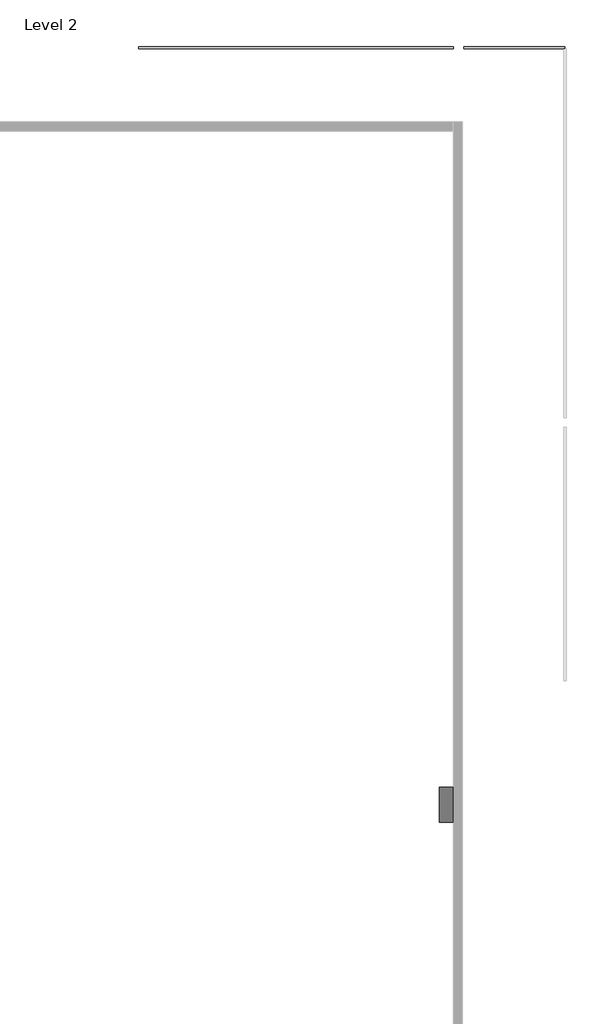
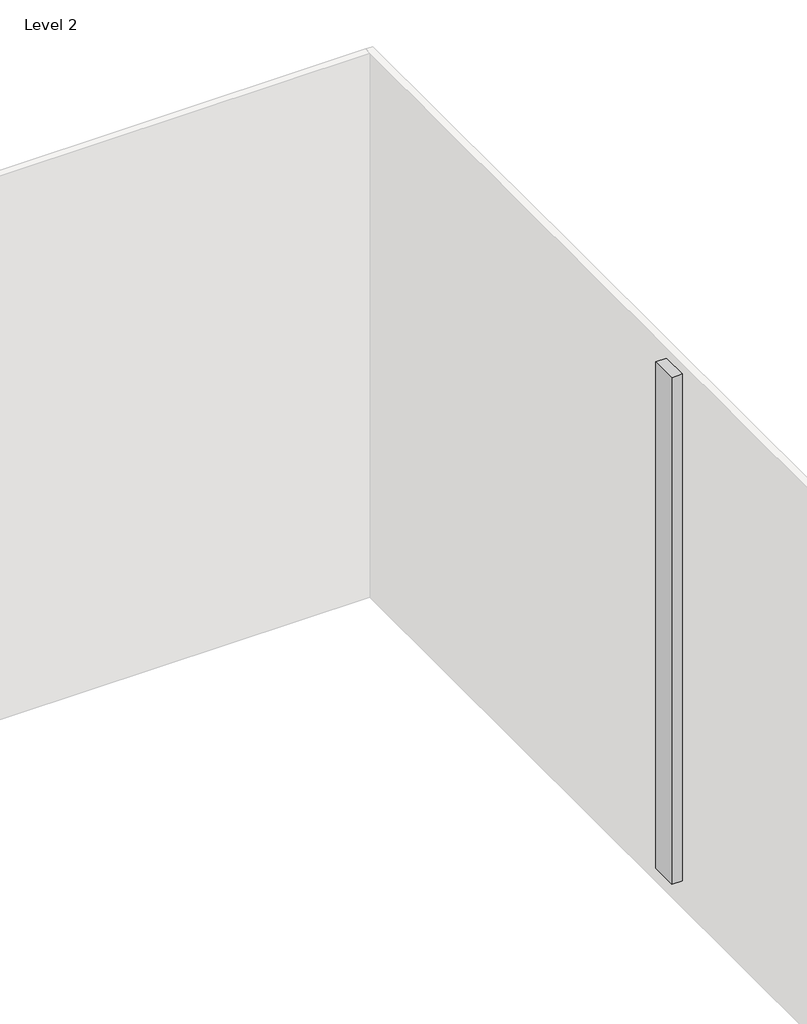
# One storey, part 5 of 5: 2 railings, 1 proxy.
"""IFC4 building model written with IfcOpenShell, lengths in millimetres."""

from ifc_helpers import new_model, si_unit, frame, origin, place, context, project, spatial, polyline, outline, extrude, transform, mapped, element, save
from components import generic_models_2_generic_models_2_fd6437b6

model = new_model("IFC4")

# Units and contexts
model_context = context("Model", 3, world=origin())
ifc_project = project(units=[si_unit("LENGTHUNIT", "METRE", prefix="MILLI")], contexts=[model_context])

# Site, building, storey
site = spatial("IfcSite", under=ifc_project)
building = spatial("IfcBuilding", under=site)
storey = spatial("IfcBuildingStorey", under=building, Name="Level 2", Elevation=3048.0)

# Proxy
placement = place(None, origin())
generic_models_2_generic_models_2_shape = generic_models_2_generic_models_2_fd6437b6(model_context)
element("IfcBuildingElementProxy", 1, Name="Generic Models 2 : Generic Models 2", ObjectType="Generic Models 2 : Generic Models 2", at=placement, inside=storey, context=model_context, shape_type="MappedRepresentation", body=[
    mapped(generic_models_2_generic_models_2_shape, transform((0.0, 0.0, 0.0), x_axis=(1.0, 0.0, 0.0), y_axis=(0.0, 1.0, 0.0), z_axis=(0.0, 0.0, 1.0))),
])

# Railings
element("IfcRailing", 2, ObjectType="Handrail - Rectangular", at=placement, inside=storey, context=model_context, shape_type="SweptSolid", body=[
    extrude(outline(polyline([(14131.9361222, 16349.0250499), (14131.9361222, 16399.8250499), (16321.4289933, 16399.8250499), (16321.4289933, 16349.0250499), (14131.9361222, 16349.0250499)])), frame((0.0, 0.0, 3911.6), z_axis=(0.0, 0.0, 1.0), x_axis=(1.0, 0.0, 0.0)), (0.0, 0.0, 1.0), 50.8),
    extrude(outline(polyline([(16256.0111222, 16364.9000499), (16256.0111222, 16383.9500499), (16275.0611222, 16383.9500499), (16275.0611222, 16364.9000499), (16256.0111222, 16364.9000499)])), frame((0.0, 0.0, 3048.0), z_axis=(0.0, 0.0, 1.0), x_axis=(1.0, 0.0, 0.0)), (0.0, 0.0, 1.0), 863.6),
    extrude(outline(polyline([(16154.4111222, 16364.9000499), (16154.4111222, 16383.9500499), (16173.4611222, 16383.9500499), (16173.4611222, 16364.9000499), (16154.4111222, 16364.9000499)])), frame((0.0, 0.0, 3048.0), z_axis=(0.0, 0.0, 1.0), x_axis=(1.0, 0.0, 0.0)), (0.0, 0.0, 1.0), 863.6),
    extrude(outline(polyline([(16052.8111222, 16364.9000499), (16052.8111222, 16383.9500499), (16071.8611222, 16383.9500499), (16071.8611222, 16364.9000499), (16052.8111222, 16364.9000499)])), frame((0.0, 0.0, 3048.0), z_axis=(0.0, 0.0, 1.0), x_axis=(1.0, 0.0, 0.0)), (0.0, 0.0, 1.0), 863.6),
    extrude(outline(polyline([(15951.2111222, 16364.9000499), (15951.2111222, 16383.9500499), (15970.2611222, 16383.9500499), (15970.2611222, 16364.9000499), (15951.2111222, 16364.9000499)])), frame((0.0, 0.0, 3048.0), z_axis=(0.0, 0.0, 1.0), x_axis=(1.0, 0.0, 0.0)), (0.0, 0.0, 1.0), 863.6),
    extrude(outline(polyline([(15849.6111222, 16364.9000499), (15849.6111222, 16383.9500499), (15868.6611222, 16383.9500499), (15868.6611222, 16364.9000499), (15849.6111222, 16364.9000499)])), frame((0.0, 0.0, 3048.0), z_axis=(0.0, 0.0, 1.0), x_axis=(1.0, 0.0, 0.0)), (0.0, 0.0, 1.0), 863.6),
    extrude(outline(polyline([(15748.0111222, 16364.9000499), (15748.0111222, 16383.9500499), (15767.0611222, 16383.9500499), (15767.0611222, 16364.9000499), (15748.0111222, 16364.9000499)])), frame((0.0, 0.0, 3048.0), z_axis=(0.0, 0.0, 1.0), x_axis=(1.0, 0.0, 0.0)), (0.0, 0.0, 1.0), 863.6),
    extrude(outline(polyline([(15646.4111222, 16364.9000499), (15646.4111222, 16383.9500499), (15665.4611222, 16383.9500499), (15665.4611222, 16364.9000499), (15646.4111222, 16364.9000499)])), frame((0.0, 0.0, 3048.0), z_axis=(0.0, 0.0, 1.0), x_axis=(1.0, 0.0, 0.0)), (0.0, 0.0, 1.0), 863.6),
    extrude(outline(polyline([(15544.8111222, 16364.9000499), (15544.8111222, 16383.9500499), (15563.8611222, 16383.9500499), (15563.8611222, 16364.9000499), (15544.8111222, 16364.9000499)])), frame((0.0, 0.0, 3048.0), z_axis=(0.0, 0.0, 1.0), x_axis=(1.0, 0.0, 0.0)), (0.0, 0.0, 1.0), 863.6),
    extrude(outline(polyline([(15443.2111222, 16364.9000499), (15443.2111222, 16383.9500499), (15462.2611222, 16383.9500499), (15462.2611222, 16364.9000499), (15443.2111222, 16364.9000499)])), frame((0.0, 0.0, 3048.0), z_axis=(0.0, 0.0, 1.0), x_axis=(1.0, 0.0, 0.0)), (0.0, 0.0, 1.0), 863.6),
    extrude(outline(polyline([(15341.6111222, 16364.9000499), (15341.6111222, 16383.9500499), (15360.6611222, 16383.9500499), (15360.6611222, 16364.9000499), (15341.6111222, 16364.9000499)])), frame((0.0, 0.0, 3048.0), z_axis=(0.0, 0.0, 1.0), x_axis=(1.0, 0.0, 0.0)), (0.0, 0.0, 1.0), 863.6),
    extrude(outline(polyline([(15240.0111222, 16364.9000499), (15240.0111222, 16383.9500499), (15259.0611222, 16383.9500499), (15259.0611222, 16364.9000499), (15240.0111222, 16364.9000499)])), frame((0.0, 0.0, 3048.0), z_axis=(0.0, 0.0, 1.0), x_axis=(1.0, 0.0, 0.0)), (0.0, 0.0, 1.0), 863.6),
    extrude(outline(polyline([(15138.4111222, 16364.9000499), (15138.4111222, 16383.9500499), (15157.4611222, 16383.9500499), (15157.4611222, 16364.9000499), (15138.4111222, 16364.9000499)])), frame((0.0, 0.0, 3048.0), z_axis=(0.0, 0.0, 1.0), x_axis=(1.0, 0.0, 0.0)), (0.0, 0.0, 1.0), 863.6),
    extrude(outline(polyline([(15036.8111222, 16364.9000499), (15036.8111222, 16383.9500499), (15055.8611222, 16383.9500499), (15055.8611222, 16364.9000499), (15036.8111222, 16364.9000499)])), frame((0.0, 0.0, 3048.0), z_axis=(0.0, 0.0, 1.0), x_axis=(1.0, 0.0, 0.0)), (0.0, 0.0, 1.0), 863.6),
    extrude(outline(polyline([(14935.2111222, 16364.9000499), (14935.2111222, 16383.9500499), (14954.2611222, 16383.9500499), (14954.2611222, 16364.9000499), (14935.2111222, 16364.9000499)])), frame((0.0, 0.0, 3048.0), z_axis=(0.0, 0.0, 1.0), x_axis=(1.0, 0.0, 0.0)), (0.0, 0.0, 1.0), 863.6),
    extrude(outline(polyline([(14833.6111222, 16364.9000499), (14833.6111222, 16383.9500499), (14852.6611222, 16383.9500499), (14852.6611222, 16364.9000499), (14833.6111222, 16364.9000499)])), frame((0.0, 0.0, 3048.0), z_axis=(0.0, 0.0, 1.0), x_axis=(1.0, 0.0, 0.0)), (0.0, 0.0, 1.0), 863.6),
    extrude(outline(polyline([(14732.0111222, 16364.9000499), (14732.0111222, 16383.9500499), (14751.0611222, 16383.9500499), (14751.0611222, 16364.9000499), (14732.0111222, 16364.9000499)])), frame((0.0, 0.0, 3048.0), z_axis=(0.0, 0.0, 1.0), x_axis=(1.0, 0.0, 0.0)), (0.0, 0.0, 1.0), 863.6),
    extrude(outline(polyline([(14630.4111222, 16364.9000499), (14630.4111222, 16383.9500499), (14649.4611222, 16383.9500499), (14649.4611222, 16364.9000499), (14630.4111222, 16364.9000499)])), frame((0.0, 0.0, 3048.0), z_axis=(0.0, 0.0, 1.0), x_axis=(1.0, 0.0, 0.0)), (0.0, 0.0, 1.0), 863.6),
    extrude(outline(polyline([(14528.8111222, 16364.9000499), (14528.8111222, 16383.9500499), (14547.8611222, 16383.9500499), (14547.8611222, 16364.9000499), (14528.8111222, 16364.9000499)])), frame((0.0, 0.0, 3048.0), z_axis=(0.0, 0.0, 1.0), x_axis=(1.0, 0.0, 0.0)), (0.0, 0.0, 1.0), 863.6),
    extrude(outline(polyline([(14427.2111222, 16364.9000499), (14427.2111222, 16383.9500499), (14446.2611222, 16383.9500499), (14446.2611222, 16364.9000499), (14427.2111222, 16364.9000499)])), frame((0.0, 0.0, 3048.0), z_axis=(0.0, 0.0, 1.0), x_axis=(1.0, 0.0, 0.0)), (0.0, 0.0, 1.0), 863.6),
    extrude(outline(polyline([(14325.6111222, 16364.9000499), (14325.6111222, 16383.9500499), (14344.6611222, 16383.9500499), (14344.6611222, 16364.9000499), (14325.6111222, 16364.9000499)])), frame((0.0, 0.0, 3048.0), z_axis=(0.0, 0.0, 1.0), x_axis=(1.0, 0.0, 0.0)), (0.0, 0.0, 1.0), 863.6),
    extrude(outline(polyline([(14224.0111222, 16364.9000499), (14224.0111222, 16383.9500499), (14243.0611222, 16383.9500499), (14243.0611222, 16364.9000499), (14224.0111222, 16364.9000499)])), frame((0.0, 0.0, 3048.0), z_axis=(0.0, 0.0, 1.0), x_axis=(1.0, 0.0, 0.0)), (0.0, 0.0, 1.0), 863.6),
    extrude(outline(polyline([(16302.3789933, 16364.9000499), (16302.3789933, 16383.9500499), (16321.4289933, 16383.9500499), (16321.4289933, 16364.9000499), (16302.3789933, 16364.9000499)])), frame((0.0, 0.0, 3048.0), z_axis=(0.0, 0.0, 1.0), x_axis=(1.0, 0.0, 0.0)), (0.0, 0.0, 1.0), 863.6),
    extrude(outline(polyline([(14131.9361222, 16364.9000499), (14131.9361222, 16383.9500499), (14150.9861222, 16383.9500499), (14150.9861222, 16364.9000499), (14131.9361222, 16364.9000499)])), frame((0.0, 0.0, 3048.0), z_axis=(0.0, 0.0, 1.0), x_axis=(1.0, 0.0, 0.0)), (0.0, 0.0, 1.0), 863.6),
])
element("IfcRailing", 3, ObjectType="Handrail - Rectangular", at=placement, inside=storey, context=model_context, shape_type="SweptSolid", body=[
    extrude(outline(polyline([(7096.1361222, 16349.0250499), (7096.1361222, 16399.8250499), (13903.3361222, 16399.8250499), (13903.3361222, 16349.0250499), (7096.1361222, 16349.0250499)])), frame((0.0, 0.0, 3911.6), z_axis=(0.0, 0.0, 1.0), x_axis=(1.0, 0.0, 0.0)), (0.0, 0.0, 1.0), 50.8),
    extrude(outline(polyline([(13792.2111222, 16364.9000499), (13792.2111222, 16383.9500499), (13811.2611222, 16383.9500499), (13811.2611222, 16364.9000499), (13792.2111222, 16364.9000499)])), frame((0.0, 0.0, 3048.0), z_axis=(0.0, 0.0, 1.0), x_axis=(1.0, 0.0, 0.0)), (0.0, 0.0, 1.0), 863.6),
    extrude(outline(polyline([(13690.6111222, 16364.9000499), (13690.6111222, 16383.9500499), (13709.6611222, 16383.9500499), (13709.6611222, 16364.9000499), (13690.6111222, 16364.9000499)])), frame((0.0, 0.0, 3048.0), z_axis=(0.0, 0.0, 1.0), x_axis=(1.0, 0.0, 0.0)), (0.0, 0.0, 1.0), 863.6),
    extrude(outline(polyline([(13589.0111222, 16364.9000499), (13589.0111222, 16383.9500499), (13608.0611222, 16383.9500499), (13608.0611222, 16364.9000499), (13589.0111222, 16364.9000499)])), frame((0.0, 0.0, 3048.0), z_axis=(0.0, 0.0, 1.0), x_axis=(1.0, 0.0, 0.0)), (0.0, 0.0, 1.0), 863.6),
    extrude(outline(polyline([(13487.4111222, 16364.9000499), (13487.4111222, 16383.9500499), (13506.4611222, 16383.9500499), (13506.4611222, 16364.9000499), (13487.4111222, 16364.9000499)])), frame((0.0, 0.0, 3048.0), z_axis=(0.0, 0.0, 1.0), x_axis=(1.0, 0.0, 0.0)), (0.0, 0.0, 1.0), 863.6),
    extrude(outline(polyline([(13385.8111222, 16364.9000499), (13385.8111222, 16383.9500499), (13404.8611222, 16383.9500499), (13404.8611222, 16364.9000499), (13385.8111222, 16364.9000499)])), frame((0.0, 0.0, 3048.0), z_axis=(0.0, 0.0, 1.0), x_axis=(1.0, 0.0, 0.0)), (0.0, 0.0, 1.0), 863.6),
    extrude(outline(polyline([(13284.2111222, 16364.9000499), (13284.2111222, 16383.9500499), (13303.2611222, 16383.9500499), (13303.2611222, 16364.9000499), (13284.2111222, 16364.9000499)])), frame((0.0, 0.0, 3048.0), z_axis=(0.0, 0.0, 1.0), x_axis=(1.0, 0.0, 0.0)), (0.0, 0.0, 1.0), 863.6),
    extrude(outline(polyline([(13182.6111222, 16364.9000499), (13182.6111222, 16383.9500499), (13201.6611222, 16383.9500499), (13201.6611222, 16364.9000499), (13182.6111222, 16364.9000499)])), frame((0.0, 0.0, 3048.0), z_axis=(0.0, 0.0, 1.0), x_axis=(1.0, 0.0, 0.0)), (0.0, 0.0, 1.0), 863.6),
    extrude(outline(polyline([(13081.0111222, 16364.9000499), (13081.0111222, 16383.9500499), (13100.0611222, 16383.9500499), (13100.0611222, 16364.9000499), (13081.0111222, 16364.9000499)])), frame((0.0, 0.0, 3048.0), z_axis=(0.0, 0.0, 1.0), x_axis=(1.0, 0.0, 0.0)), (0.0, 0.0, 1.0), 863.6),
    extrude(outline(polyline([(12979.4111222, 16364.9000499), (12979.4111222, 16383.9500499), (12998.4611222, 16383.9500499), (12998.4611222, 16364.9000499), (12979.4111222, 16364.9000499)])), frame((0.0, 0.0, 3048.0), z_axis=(0.0, 0.0, 1.0), x_axis=(1.0, 0.0, 0.0)), (0.0, 0.0, 1.0), 863.6),
    extrude(outline(polyline([(12877.8111222, 16364.9000499), (12877.8111222, 16383.9500499), (12896.8611222, 16383.9500499), (12896.8611222, 16364.9000499), (12877.8111222, 16364.9000499)])), frame((0.0, 0.0, 3048.0), z_axis=(0.0, 0.0, 1.0), x_axis=(1.0, 0.0, 0.0)), (0.0, 0.0, 1.0), 863.6),
    extrude(outline(polyline([(12776.2111222, 16364.9000499), (12776.2111222, 16383.9500499), (12795.2611222, 16383.9500499), (12795.2611222, 16364.9000499), (12776.2111222, 16364.9000499)])), frame((0.0, 0.0, 3048.0), z_axis=(0.0, 0.0, 1.0), x_axis=(1.0, 0.0, 0.0)), (0.0, 0.0, 1.0), 863.6),
    extrude(outline(polyline([(12674.6111222, 16364.9000499), (12674.6111222, 16383.9500499), (12693.6611222, 16383.9500499), (12693.6611222, 16364.9000499), (12674.6111222, 16364.9000499)])), frame((0.0, 0.0, 3048.0), z_axis=(0.0, 0.0, 1.0), x_axis=(1.0, 0.0, 0.0)), (0.0, 0.0, 1.0), 863.6),
    extrude(outline(polyline([(12573.0111222, 16364.9000499), (12573.0111222, 16383.9500499), (12592.0611222, 16383.9500499), (12592.0611222, 16364.9000499), (12573.0111222, 16364.9000499)])), frame((0.0, 0.0, 3048.0), z_axis=(0.0, 0.0, 1.0), x_axis=(1.0, 0.0, 0.0)), (0.0, 0.0, 1.0), 863.6),
    extrude(outline(polyline([(12471.4111222, 16364.9000499), (12471.4111222, 16383.9500499), (12490.4611222, 16383.9500499), (12490.4611222, 16364.9000499), (12471.4111222, 16364.9000499)])), frame((0.0, 0.0, 3048.0), z_axis=(0.0, 0.0, 1.0), x_axis=(1.0, 0.0, 0.0)), (0.0, 0.0, 1.0), 863.6),
    extrude(outline(polyline([(12369.8111222, 16364.9000499), (12369.8111222, 16383.9500499), (12388.8611222, 16383.9500499), (12388.8611222, 16364.9000499), (12369.8111222, 16364.9000499)])), frame((0.0, 0.0, 3048.0), z_axis=(0.0, 0.0, 1.0), x_axis=(1.0, 0.0, 0.0)), (0.0, 0.0, 1.0), 863.6),
    extrude(outline(polyline([(12268.2111222, 16364.9000499), (12268.2111222, 16383.9500499), (12287.2611222, 16383.9500499), (12287.2611222, 16364.9000499), (12268.2111222, 16364.9000499)])), frame((0.0, 0.0, 3048.0), z_axis=(0.0, 0.0, 1.0), x_axis=(1.0, 0.0, 0.0)), (0.0, 0.0, 1.0), 863.6),
    extrude(outline(polyline([(12166.6111222, 16364.9000499), (12166.6111222, 16383.9500499), (12185.6611222, 16383.9500499), (12185.6611222, 16364.9000499), (12166.6111222, 16364.9000499)])), frame((0.0, 0.0, 3048.0), z_axis=(0.0, 0.0, 1.0), x_axis=(1.0, 0.0, 0.0)), (0.0, 0.0, 1.0), 863.6),
    extrude(outline(polyline([(12065.0111222, 16364.9000499), (12065.0111222, 16383.9500499), (12084.0611222, 16383.9500499), (12084.0611222, 16364.9000499), (12065.0111222, 16364.9000499)])), frame((0.0, 0.0, 3048.0), z_axis=(0.0, 0.0, 1.0), x_axis=(1.0, 0.0, 0.0)), (0.0, 0.0, 1.0), 863.6),
    extrude(outline(polyline([(11963.4111222, 16364.9000499), (11963.4111222, 16383.9500499), (11982.4611222, 16383.9500499), (11982.4611222, 16364.9000499), (11963.4111222, 16364.9000499)])), frame((0.0, 0.0, 3048.0), z_axis=(0.0, 0.0, 1.0), x_axis=(1.0, 0.0, 0.0)), (0.0, 0.0, 1.0), 863.6),
    extrude(outline(polyline([(11861.8111222, 16364.9000499), (11861.8111222, 16383.9500499), (11880.8611222, 16383.9500499), (11880.8611222, 16364.9000499), (11861.8111222, 16364.9000499)])), frame((0.0, 0.0, 3048.0), z_axis=(0.0, 0.0, 1.0), x_axis=(1.0, 0.0, 0.0)), (0.0, 0.0, 1.0), 863.6),
    extrude(outline(polyline([(11760.2111222, 16364.9000499), (11760.2111222, 16383.9500499), (11779.2611222, 16383.9500499), (11779.2611222, 16364.9000499), (11760.2111222, 16364.9000499)])), frame((0.0, 0.0, 3048.0), z_axis=(0.0, 0.0, 1.0), x_axis=(1.0, 0.0, 0.0)), (0.0, 0.0, 1.0), 863.6),
    extrude(outline(polyline([(11658.6111222, 16364.9000499), (11658.6111222, 16383.9500499), (11677.6611222, 16383.9500499), (11677.6611222, 16364.9000499), (11658.6111222, 16364.9000499)])), frame((0.0, 0.0, 3048.0), z_axis=(0.0, 0.0, 1.0), x_axis=(1.0, 0.0, 0.0)), (0.0, 0.0, 1.0), 863.6),
    extrude(outline(polyline([(11557.0111222, 16364.9000499), (11557.0111222, 16383.9500499), (11576.0611222, 16383.9500499), (11576.0611222, 16364.9000499), (11557.0111222, 16364.9000499)])), frame((0.0, 0.0, 3048.0), z_axis=(0.0, 0.0, 1.0), x_axis=(1.0, 0.0, 0.0)), (0.0, 0.0, 1.0), 863.6),
    extrude(outline(polyline([(11455.4111222, 16364.9000499), (11455.4111222, 16383.9500499), (11474.4611222, 16383.9500499), (11474.4611222, 16364.9000499), (11455.4111222, 16364.9000499)])), frame((0.0, 0.0, 3048.0), z_axis=(0.0, 0.0, 1.0), x_axis=(1.0, 0.0, 0.0)), (0.0, 0.0, 1.0), 863.6),
    extrude(outline(polyline([(11353.8111222, 16364.9000499), (11353.8111222, 16383.9500499), (11372.8611222, 16383.9500499), (11372.8611222, 16364.9000499), (11353.8111222, 16364.9000499)])), frame((0.0, 0.0, 3048.0), z_axis=(0.0, 0.0, 1.0), x_axis=(1.0, 0.0, 0.0)), (0.0, 0.0, 1.0), 863.6),
    extrude(outline(polyline([(11252.2111222, 16364.9000499), (11252.2111222, 16383.9500499), (11271.2611222, 16383.9500499), (11271.2611222, 16364.9000499), (11252.2111222, 16364.9000499)])), frame((0.0, 0.0, 3048.0), z_axis=(0.0, 0.0, 1.0), x_axis=(1.0, 0.0, 0.0)), (0.0, 0.0, 1.0), 863.6),
    extrude(outline(polyline([(11150.6111222, 16364.9000499), (11150.6111222, 16383.9500499), (11169.6611222, 16383.9500499), (11169.6611222, 16364.9000499), (11150.6111222, 16364.9000499)])), frame((0.0, 0.0, 3048.0), z_axis=(0.0, 0.0, 1.0), x_axis=(1.0, 0.0, 0.0)), (0.0, 0.0, 1.0), 863.6),
    extrude(outline(polyline([(11049.0111222, 16364.9000499), (11049.0111222, 16383.9500499), (11068.0611222, 16383.9500499), (11068.0611222, 16364.9000499), (11049.0111222, 16364.9000499)])), frame((0.0, 0.0, 3048.0), z_axis=(0.0, 0.0, 1.0), x_axis=(1.0, 0.0, 0.0)), (0.0, 0.0, 1.0), 863.6),
    extrude(outline(polyline([(10947.4111222, 16364.9000499), (10947.4111222, 16383.9500499), (10966.4611222, 16383.9500499), (10966.4611222, 16364.9000499), (10947.4111222, 16364.9000499)])), frame((0.0, 0.0, 3048.0), z_axis=(0.0, 0.0, 1.0), x_axis=(1.0, 0.0, 0.0)), (0.0, 0.0, 1.0), 863.6),
    extrude(outline(polyline([(10845.8111222, 16364.9000499), (10845.8111222, 16383.9500499), (10864.8611222, 16383.9500499), (10864.8611222, 16364.9000499), (10845.8111222, 16364.9000499)])), frame((0.0, 0.0, 3048.0), z_axis=(0.0, 0.0, 1.0), x_axis=(1.0, 0.0, 0.0)), (0.0, 0.0, 1.0), 863.6),
    extrude(outline(polyline([(10744.2111222, 16364.9000499), (10744.2111222, 16383.9500499), (10763.2611222, 16383.9500499), (10763.2611222, 16364.9000499), (10744.2111222, 16364.9000499)])), frame((0.0, 0.0, 3048.0), z_axis=(0.0, 0.0, 1.0), x_axis=(1.0, 0.0, 0.0)), (0.0, 0.0, 1.0), 863.6),
    extrude(outline(polyline([(10642.6111222, 16364.9000499), (10642.6111222, 16383.9500499), (10661.6611222, 16383.9500499), (10661.6611222, 16364.9000499), (10642.6111222, 16364.9000499)])), frame((0.0, 0.0, 3048.0), z_axis=(0.0, 0.0, 1.0), x_axis=(1.0, 0.0, 0.0)), (0.0, 0.0, 1.0), 863.6),
    extrude(outline(polyline([(10541.0111222, 16364.9000499), (10541.0111222, 16383.9500499), (10560.0611222, 16383.9500499), (10560.0611222, 16364.9000499), (10541.0111222, 16364.9000499)])), frame((0.0, 0.0, 3048.0), z_axis=(0.0, 0.0, 1.0), x_axis=(1.0, 0.0, 0.0)), (0.0, 0.0, 1.0), 863.6),
    extrude(outline(polyline([(10439.4111222, 16364.9000499), (10439.4111222, 16383.9500499), (10458.4611222, 16383.9500499), (10458.4611222, 16364.9000499), (10439.4111222, 16364.9000499)])), frame((0.0, 0.0, 3048.0), z_axis=(0.0, 0.0, 1.0), x_axis=(1.0, 0.0, 0.0)), (0.0, 0.0, 1.0), 863.6),
    extrude(outline(polyline([(10337.8111222, 16364.9000499), (10337.8111222, 16383.9500499), (10356.8611222, 16383.9500499), (10356.8611222, 16364.9000499), (10337.8111222, 16364.9000499)])), frame((0.0, 0.0, 3048.0), z_axis=(0.0, 0.0, 1.0), x_axis=(1.0, 0.0, 0.0)), (0.0, 0.0, 1.0), 863.6),
    extrude(outline(polyline([(10236.2111222, 16364.9000499), (10236.2111222, 16383.9500499), (10255.2611222, 16383.9500499), (10255.2611222, 16364.9000499), (10236.2111222, 16364.9000499)])), frame((0.0, 0.0, 3048.0), z_axis=(0.0, 0.0, 1.0), x_axis=(1.0, 0.0, 0.0)), (0.0, 0.0, 1.0), 863.6),
    extrude(outline(polyline([(10134.6111222, 16364.9000499), (10134.6111222, 16383.9500499), (10153.6611222, 16383.9500499), (10153.6611222, 16364.9000499), (10134.6111222, 16364.9000499)])), frame((0.0, 0.0, 3048.0), z_axis=(0.0, 0.0, 1.0), x_axis=(1.0, 0.0, 0.0)), (0.0, 0.0, 1.0), 863.6),
    extrude(outline(polyline([(10033.0111222, 16364.9000499), (10033.0111222, 16383.9500499), (10052.0611222, 16383.9500499), (10052.0611222, 16364.9000499), (10033.0111222, 16364.9000499)])), frame((0.0, 0.0, 3048.0), z_axis=(0.0, 0.0, 1.0), x_axis=(1.0, 0.0, 0.0)), (0.0, 0.0, 1.0), 863.6),
    extrude(outline(polyline([(9931.4111222, 16364.9000499), (9931.4111222, 16383.9500499), (9950.4611222, 16383.9500499), (9950.4611222, 16364.9000499), (9931.4111222, 16364.9000499)])), frame((0.0, 0.0, 3048.0), z_axis=(0.0, 0.0, 1.0), x_axis=(1.0, 0.0, 0.0)), (0.0, 0.0, 1.0), 863.6),
    extrude(outline(polyline([(9829.8111222, 16364.9000499), (9829.8111222, 16383.9500499), (9848.8611222, 16383.9500499), (9848.8611222, 16364.9000499), (9829.8111222, 16364.9000499)])), frame((0.0, 0.0, 3048.0), z_axis=(0.0, 0.0, 1.0), x_axis=(1.0, 0.0, 0.0)), (0.0, 0.0, 1.0), 863.6),
    extrude(outline(polyline([(9728.2111222, 16364.9000499), (9728.2111222, 16383.9500499), (9747.2611222, 16383.9500499), (9747.2611222, 16364.9000499), (9728.2111222, 16364.9000499)])), frame((0.0, 0.0, 3048.0), z_axis=(0.0, 0.0, 1.0), x_axis=(1.0, 0.0, 0.0)), (0.0, 0.0, 1.0), 863.6),
    extrude(outline(polyline([(9626.6111222, 16364.9000499), (9626.6111222, 16383.9500499), (9645.6611222, 16383.9500499), (9645.6611222, 16364.9000499), (9626.6111222, 16364.9000499)])), frame((0.0, 0.0, 3048.0), z_axis=(0.0, 0.0, 1.0), x_axis=(1.0, 0.0, 0.0)), (0.0, 0.0, 1.0), 863.6),
    extrude(outline(polyline([(9525.0111222, 16364.9000499), (9525.0111222, 16383.9500499), (9544.0611222, 16383.9500499), (9544.0611222, 16364.9000499), (9525.0111222, 16364.9000499)])), frame((0.0, 0.0, 3048.0), z_axis=(0.0, 0.0, 1.0), x_axis=(1.0, 0.0, 0.0)), (0.0, 0.0, 1.0), 863.6),
    extrude(outline(polyline([(9423.4111222, 16364.9000499), (9423.4111222, 16383.9500499), (9442.4611222, 16383.9500499), (9442.4611222, 16364.9000499), (9423.4111222, 16364.9000499)])), frame((0.0, 0.0, 3048.0), z_axis=(0.0, 0.0, 1.0), x_axis=(1.0, 0.0, 0.0)), (0.0, 0.0, 1.0), 863.6),
    extrude(outline(polyline([(9321.8111222, 16364.9000499), (9321.8111222, 16383.9500499), (9340.8611222, 16383.9500499), (9340.8611222, 16364.9000499), (9321.8111222, 16364.9000499)])), frame((0.0, 0.0, 3048.0), z_axis=(0.0, 0.0, 1.0), x_axis=(1.0, 0.0, 0.0)), (0.0, 0.0, 1.0), 863.6),
    extrude(outline(polyline([(9220.2111222, 16364.9000499), (9220.2111222, 16383.9500499), (9239.2611222, 16383.9500499), (9239.2611222, 16364.9000499), (9220.2111222, 16364.9000499)])), frame((0.0, 0.0, 3048.0), z_axis=(0.0, 0.0, 1.0), x_axis=(1.0, 0.0, 0.0)), (0.0, 0.0, 1.0), 863.6),
    extrude(outline(polyline([(9118.6111222, 16364.9000499), (9118.6111222, 16383.9500499), (9137.6611222, 16383.9500499), (9137.6611222, 16364.9000499), (9118.6111222, 16364.9000499)])), frame((0.0, 0.0, 3048.0), z_axis=(0.0, 0.0, 1.0), x_axis=(1.0, 0.0, 0.0)), (0.0, 0.0, 1.0), 863.6),
    extrude(outline(polyline([(9017.0111222, 16364.9000499), (9017.0111222, 16383.9500499), (9036.0611222, 16383.9500499), (9036.0611222, 16364.9000499), (9017.0111222, 16364.9000499)])), frame((0.0, 0.0, 3048.0), z_axis=(0.0, 0.0, 1.0), x_axis=(1.0, 0.0, 0.0)), (0.0, 0.0, 1.0), 863.6),
    extrude(outline(polyline([(8915.4111222, 16364.9000499), (8915.4111222, 16383.9500499), (8934.4611222, 16383.9500499), (8934.4611222, 16364.9000499), (8915.4111222, 16364.9000499)])), frame((0.0, 0.0, 3048.0), z_axis=(0.0, 0.0, 1.0), x_axis=(1.0, 0.0, 0.0)), (0.0, 0.0, 1.0), 863.6),
    extrude(outline(polyline([(8813.8111222, 16364.9000499), (8813.8111222, 16383.9500499), (8832.8611222, 16383.9500499), (8832.8611222, 16364.9000499), (8813.8111222, 16364.9000499)])), frame((0.0, 0.0, 3048.0), z_axis=(0.0, 0.0, 1.0), x_axis=(1.0, 0.0, 0.0)), (0.0, 0.0, 1.0), 863.6),
    extrude(outline(polyline([(8712.2111222, 16364.9000499), (8712.2111222, 16383.9500499), (8731.2611222, 16383.9500499), (8731.2611222, 16364.9000499), (8712.2111222, 16364.9000499)])), frame((0.0, 0.0, 3048.0), z_axis=(0.0, 0.0, 1.0), x_axis=(1.0, 0.0, 0.0)), (0.0, 0.0, 1.0), 863.6),
    extrude(outline(polyline([(8610.6111222, 16364.9000499), (8610.6111222, 16383.9500499), (8629.6611222, 16383.9500499), (8629.6611222, 16364.9000499), (8610.6111222, 16364.9000499)])), frame((0.0, 0.0, 3048.0), z_axis=(0.0, 0.0, 1.0), x_axis=(1.0, 0.0, 0.0)), (0.0, 0.0, 1.0), 863.6),
    extrude(outline(polyline([(8509.0111222, 16364.9000499), (8509.0111222, 16383.9500499), (8528.0611222, 16383.9500499), (8528.0611222, 16364.9000499), (8509.0111222, 16364.9000499)])), frame((0.0, 0.0, 3048.0), z_axis=(0.0, 0.0, 1.0), x_axis=(1.0, 0.0, 0.0)), (0.0, 0.0, 1.0), 863.6),
    extrude(outline(polyline([(8407.4111222, 16364.9000499), (8407.4111222, 16383.9500499), (8426.4611222, 16383.9500499), (8426.4611222, 16364.9000499), (8407.4111222, 16364.9000499)])), frame((0.0, 0.0, 3048.0), z_axis=(0.0, 0.0, 1.0), x_axis=(1.0, 0.0, 0.0)), (0.0, 0.0, 1.0), 863.6),
    extrude(outline(polyline([(8305.8111222, 16364.9000499), (8305.8111222, 16383.9500499), (8324.8611222, 16383.9500499), (8324.8611222, 16364.9000499), (8305.8111222, 16364.9000499)])), frame((0.0, 0.0, 3048.0), z_axis=(0.0, 0.0, 1.0), x_axis=(1.0, 0.0, 0.0)), (0.0, 0.0, 1.0), 863.6),
    extrude(outline(polyline([(8204.2111222, 16364.9000499), (8204.2111222, 16383.9500499), (8223.2611222, 16383.9500499), (8223.2611222, 16364.9000499), (8204.2111222, 16364.9000499)])), frame((0.0, 0.0, 3048.0), z_axis=(0.0, 0.0, 1.0), x_axis=(1.0, 0.0, 0.0)), (0.0, 0.0, 1.0), 863.6),
    extrude(outline(polyline([(8102.6111222, 16364.9000499), (8102.6111222, 16383.9500499), (8121.6611222, 16383.9500499), (8121.6611222, 16364.9000499), (8102.6111222, 16364.9000499)])), frame((0.0, 0.0, 3048.0), z_axis=(0.0, 0.0, 1.0), x_axis=(1.0, 0.0, 0.0)), (0.0, 0.0, 1.0), 863.6),
    extrude(outline(polyline([(8001.0111222, 16364.9000499), (8001.0111222, 16383.9500499), (8020.0611222, 16383.9500499), (8020.0611222, 16364.9000499), (8001.0111222, 16364.9000499)])), frame((0.0, 0.0, 3048.0), z_axis=(0.0, 0.0, 1.0), x_axis=(1.0, 0.0, 0.0)), (0.0, 0.0, 1.0), 863.6),
    extrude(outline(polyline([(7899.4111222, 16364.9000499), (7899.4111222, 16383.9500499), (7918.4611222, 16383.9500499), (7918.4611222, 16364.9000499), (7899.4111222, 16364.9000499)])), frame((0.0, 0.0, 3048.0), z_axis=(0.0, 0.0, 1.0), x_axis=(1.0, 0.0, 0.0)), (0.0, 0.0, 1.0), 863.6),
    extrude(outline(polyline([(7797.8111222, 16364.9000499), (7797.8111222, 16383.9500499), (7816.8611222, 16383.9500499), (7816.8611222, 16364.9000499), (7797.8111222, 16364.9000499)])), frame((0.0, 0.0, 3048.0), z_axis=(0.0, 0.0, 1.0), x_axis=(1.0, 0.0, 0.0)), (0.0, 0.0, 1.0), 863.6),
    extrude(outline(polyline([(7696.2111222, 16364.9000499), (7696.2111222, 16383.9500499), (7715.2611222, 16383.9500499), (7715.2611222, 16364.9000499), (7696.2111222, 16364.9000499)])), frame((0.0, 0.0, 3048.0), z_axis=(0.0, 0.0, 1.0), x_axis=(1.0, 0.0, 0.0)), (0.0, 0.0, 1.0), 863.6),
    extrude(outline(polyline([(7594.6111222, 16364.9000499), (7594.6111222, 16383.9500499), (7613.6611222, 16383.9500499), (7613.6611222, 16364.9000499), (7594.6111222, 16364.9000499)])), frame((0.0, 0.0, 3048.0), z_axis=(0.0, 0.0, 1.0), x_axis=(1.0, 0.0, 0.0)), (0.0, 0.0, 1.0), 863.6),
    extrude(outline(polyline([(7493.0111222, 16364.9000499), (7493.0111222, 16383.9500499), (7512.0611222, 16383.9500499), (7512.0611222, 16364.9000499), (7493.0111222, 16364.9000499)])), frame((0.0, 0.0, 3048.0), z_axis=(0.0, 0.0, 1.0), x_axis=(1.0, 0.0, 0.0)), (0.0, 0.0, 1.0), 863.6),
    extrude(outline(polyline([(7391.4111222, 16364.9000499), (7391.4111222, 16383.9500499), (7410.4611222, 16383.9500499), (7410.4611222, 16364.9000499), (7391.4111222, 16364.9000499)])), frame((0.0, 0.0, 3048.0), z_axis=(0.0, 0.0, 1.0), x_axis=(1.0, 0.0, 0.0)), (0.0, 0.0, 1.0), 863.6),
    extrude(outline(polyline([(7289.8111222, 16364.9000499), (7289.8111222, 16383.9500499), (7308.8611222, 16383.9500499), (7308.8611222, 16364.9000499), (7289.8111222, 16364.9000499)])), frame((0.0, 0.0, 3048.0), z_axis=(0.0, 0.0, 1.0), x_axis=(1.0, 0.0, 0.0)), (0.0, 0.0, 1.0), 863.6),
    extrude(outline(polyline([(7188.2111222, 16364.9000499), (7188.2111222, 16383.9500499), (7207.2611222, 16383.9500499), (7207.2611222, 16364.9000499), (7188.2111222, 16364.9000499)])), frame((0.0, 0.0, 3048.0), z_axis=(0.0, 0.0, 1.0), x_axis=(1.0, 0.0, 0.0)), (0.0, 0.0, 1.0), 863.6),
    extrude(outline(polyline([(13884.2861222, 16364.9000499), (13884.2861222, 16383.9500499), (13903.3361222, 16383.9500499), (13903.3361222, 16364.9000499), (13884.2861222, 16364.9000499)])), frame((0.0, 0.0, 3048.0), z_axis=(0.0, 0.0, 1.0), x_axis=(1.0, 0.0, 0.0)), (0.0, 0.0, 1.0), 863.6),
    extrude(outline(polyline([(7096.1361222, 16364.9000499), (7096.1361222, 16383.9500499), (7115.1861222, 16383.9500499), (7115.1861222, 16364.9000499), (7096.1361222, 16364.9000499)])), frame((0.0, 0.0, 3048.0), z_axis=(0.0, 0.0, 1.0), x_axis=(1.0, 0.0, 0.0)), (0.0, 0.0, 1.0), 863.6),
])

save(model, "model.ifc")

# Revit data of these elements
# Type "Handrail - Rectangular"
#   Assembly Code = "C2010400"
#   built-in parameter 1008612 = 0.0416667 (stored number, unit not read)
#   built-in parameter 1008611 = 0.0416667 (stored number, unit not read)
#   built-in parameter 1008609 = 0.333333 (stored number, unit not read)
#   built-in parameter 1008604 = 0.166667 (stored number, unit not read)
#   built-in parameter 1008603 = 0.166667 (stored number, unit not read)
#   Railing Height = 3' - 0"
#   built-in parameter 1008630 = 2
#   built-in parameter 1008610 = 2
#   built-in parameter 1008618 = Baluster - Square : 3/4"
# Element 1 (IfcBuildingElementProxy, "Generic Models 2 : Generic Models 2")
#   Phase Created = New Construction
# Elements 2, 3 (IfcRailing, "Handrail - Rectangular")
#   Phase Created = New Construction
